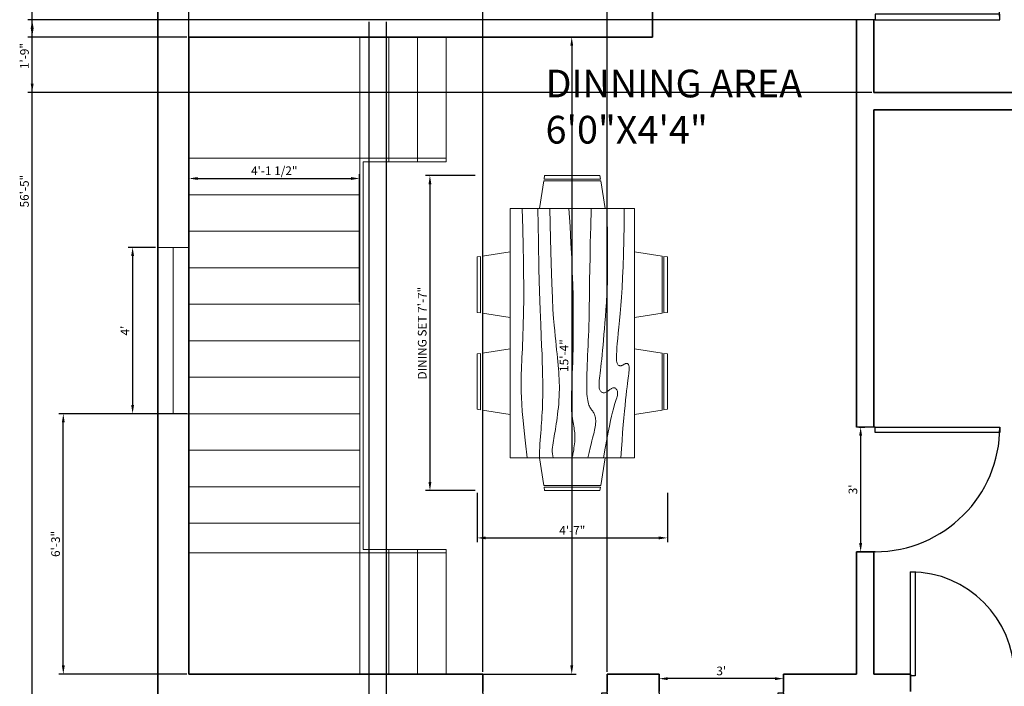
# Model space of a CAD drawing. Units: inches. Extents: x 3715 to 4224, y 2597 to 3354.
# Tile 2 of 5: x 3717 to 4001, y 2830 to 3023. Entities that reach past the tile are written whole.
import ezdxf

# ---------------------------------------------------------------- set-up
doc = ezdxf.new("R2010")
doc.units = ezdxf.units.IN
for name, color, linetype, lineweight in [('A-AREA-IDEN', 4, 'Continuous', 25), ('A-FLOR-STRS', 7, 'Continuous', 18), ('A-WALL', 7, 'Continuous', 35), ('DIM', 1, 'Continuous', 18), ('DOOR', 3, 'Continuous', 25), ('FURNITURES', 30, 'Continuous', 18), ('WINDOW', 6, 'Continuous', 20)]:
    doc.layers.add(name, color=color, linetype=linetype, lineweight=lineweight)
doc.styles.get("Standard").update_dxf_attribs({"font": 'arial.ttf'})
doc.dimstyles.new('ISO-25', dxfattribs={"dimtxt": 2.5, "dimasz": 2.5, "dimexe": 1.25, "dimexo": 0.625, "dimtad": 1, "dimlunit": 3, "dimtxsty": 'Standard', "dimcen": 2.5, "dimadec": 0, "dimazin": 0, "dimtfac": 1, "dimtmove": 0, "dimatfit": 3, "dimfxl": 1, "dimarcsym": 0})

# ---------------------------------------------------------------- blocks, each defined once
blk = doc.blocks.new('*U3')
for p, q in [((-40, 0), (-40, 6)), ((0, 0), (0, 6))]:
    blk.add_line(p, q)
blk.add_lwpolyline([(0, 0), (0, -40), (-1.75, -40), (-1.75, 0)], close=True)
blk.add_arc((0, 0), 40, 180, 270)
blk = doc.blocks.new('*U2')
for p, q in [((0, 0), (0, -6)), ((40, 0), (40, -6))]:
    blk.add_line(p, q)
blk.add_lwpolyline([(0, 0), (0, 40), (1.75, 40), (1.75, 0)], close=True)
blk.add_arc((0, 0), 40, 0, 90)
blk = doc.blocks.new('*U4')
for p, q in [((0, 0), (0, -6)), ((-40, 0), (-40, -6))]:
    blk.add_line(p, q)
blk.add_lwpolyline([(0, 0), (0, 40), (-1.75, 40), (-1.75, 0)], close=True)
blk.add_arc((0, 0), 40, 90, 180)
blk = doc.blocks.new('Dining Set - 36 x 72 in.')
for p, q in [((-22.2343, 26.00059), (-23.4847, 17.99762)), ((-22.2304, 26), (-5.7608, 26)), ((-22, 27.5), (-22.1562, 26.50042)), ((-5.8416, 26.5), (-22.1534, 26.5)), ((-22, 27.5), (-6, 27.5)), ((-5.8437, 26.49966), (-6, 27.5)), ((-4.5152, 17.99762), (-5.7655, 25.99926)), ((5.7657, 26.00059), (4.5153, 17.99762)), ((5.7696, 26), (22.2392, 26)), ((6, 27.5), (5.8438, 26.50042)), ((22.1584, 26.5), (5.8466, 26.5)), ((6, 27.5), (22, 27.5)), ((22.1563, 26.49966), (22, 27.5)), ((23.4848, 17.99762), (22.2345, 25.99926)), ((36, 18), (-36, 18)), ((-36, 18), (-36, -18)), ((36, -18), (36, 18)), ((-44.0006, 8.23428), (-35.9976, 9.48474)), ((44.0006, 8.23428), (35.9976, 9.48474)), ((-45.5, 8), (-44.5004, 8.15617)), ((-45.5, 8), (-45.5, -8)), ((-44.5, -8.15843), (-44.5, 8.15338)), ((-44, 8.23041), (-44, -8.23915)), ((44, 8.23041), (44, -8.23915)), ((44.5, -8.15843), (44.5, 8.15338)), ((45.5, 8), (44.5005, 8.15617)), ((45.5, 8), (45.5, -8)), ((-44.4997, -8.15631), (-45.5, -8)), ((-35.9976, -9.48476), (-43.9993, -8.2345)), ((35.9976, -9.48476), (43.9993, -8.2345)), ((44.4997, -8.15631), (45.5, -8)), ((-36, -18), (36, -18)), ((-22.2343, -26.0006), (-23.4847, -17.99762)), ((-4.5152, -17.99762), (-5.7655, -25.99928)), ((5.7657, -26.0006), (4.5153, -17.99762)), ((23.4848, -17.99762), (22.2345, -25.99928)), ((-22.2304, -26), (-5.7608, -26)), ((-22, -27.5), (-22.1562, -26.50044)), ((-5.8416, -26.5), (-22.1534, -26.5)), ((-22, -27.5), (-6, -27.5)), ((-5.8437, -26.49967), (-6, -27.5)), ((5.7696, -26), (22.2392, -26)), ((6, -27.5), (5.8438, -26.50044)), ((22.1584, -26.5), (5.8466, -26.5)), ((6, -27.5), (22, -27.5)), ((22.1563, -26.49967), (22, -27.5))]:
    blk.add_line(p, q)
for points in [[(-36, 15), (-31.1772, 14.97754), (-26.8079, 14.91406), (-22.8538, 14.81543), (-19.276, 14.6875), (-16.0362, 14.53613), (-13.0957, 14.36718), (-10.4159, 14.18652), (-7.9583, 14), (-5.6904, 13.81315), (-3.6035, 13.63021), (-1.6954, 13.45508), (0.0365, 13.29166), (1.5945, 13.14388), (2.9811, 13.01562), (4.1988, 12.9108), (5.25, 12.83333), (6.1393, 12.78613), (6.8802, 12.76823), (7.4883, 12.77767), (7.9792, 12.8125), (8.3685, 12.87077), (8.6719, 12.95052), (8.9049, 13.0498), (9.0833, 13.16666), (9.2205, 13.29899), (9.3216, 13.44401), (9.3895, 13.59879), (9.4271, 13.76041), (9.4373, 13.92594), (9.4232, 14.09245), (9.3875, 14.257), (9.3333, 14.41666), (9.2638, 14.56917), (9.1836, 14.71484), (9.0975, 14.85465), (9.0104, 14.98958), (8.9272, 15.1206), (8.8529, 15.2487), (8.7922, 15.37483), (8.75, 15.5), (8.7305, 15.62467), (8.7344, 15.74739), (8.7617, 15.86621), (8.8125, 15.97916), (8.8867, 16.08431), (8.9844, 16.17968), (9.1055, 16.26334), (9.25, 16.33333), (9.4189, 16.38802), (9.6172, 16.42708), (9.8506, 16.45052), (10.125, 16.45833), (10.4463, 16.45052), (10.8203, 16.42708), (11.2529, 16.38802), (11.75, 16.33333), (12.3184, 16.26318), (12.9694, 16.17838), (13.7151, 16.07991), (14.5677, 15.96875), (15.5395, 15.84586), (16.6426, 15.71224), (17.8893, 15.56884), (19.2917, 15.41666), (20.859, 15.25667), (22.5879, 15.08984), (24.4721, 14.91715), (26.5052, 14.73958), (28.6809, 14.5581), (30.9929, 14.3737), (33.4347, 14.18733), (36, 14)], [(-36, 10), (-28.9766, 10.14274), (-23.1725, 10.20442), (-18.4241, 10.19775), (-14.5677, 10.13541), (-11.4399, 10.03011), (-8.877, 9.89453), (-6.7154, 9.74137), (-4.7917, 9.58333), (-2.9698, 9.43082), (-1.2246, 9.28515), (0.4415, 9.14534), (2.026, 9.01041), (3.5266, 8.87939), (4.9408, 8.7513), (6.266, 8.62516), (7.5, 8.5), (8.6411, 8.37549), (9.6914, 8.2539), (10.6538, 8.13818), (11.5312, 8.03125), (12.3267, 7.93603), (13.043, 7.85547), (13.6831, 7.79248), (14.25, 7.75), (14.7471, 7.7303), (15.1797, 7.73307), (15.5537, 7.75732), (15.875, 7.80208), (16.1494, 7.86637), (16.3828, 7.94922), (16.5811, 8.04964), (16.75, 8.16666), (16.8944, 8.29915), (17.0143, 8.44531), (17.1089, 8.60319), (17.1771, 8.77083), (17.218, 8.94629), (17.2305, 9.1276), (17.2137, 9.31282), (17.1667, 9.5), (17.0895, 9.6875), (16.987, 9.875), (16.8649, 10.0625), (16.7292, 10.25), (16.5856, 10.4375), (16.4401, 10.625), (16.2985, 10.8125), (16.1667, 11), (16.05, 11.18733), (15.9518, 11.3737), (15.8752, 11.5581), (15.8229, 11.73958), (15.798, 11.91715), (15.8034, 12.08984), (15.842, 12.25667), (15.9167, 12.41666), (16.0295, 12.56836), (16.1784, 12.70833), (16.3605, 12.83268), (16.5729, 12.9375), (16.8127, 13.01888), (17.0768, 13.07291), (17.3625, 13.0957), (17.6667, 13.08333), (17.9894, 13.03312), (18.3418, 12.94726), (18.7382, 12.82918), (19.1927, 12.68229), (19.7195, 12.51001), (20.3327, 12.31575), (21.0465, 12.10294), (21.875, 11.875), (22.8357, 11.63354), (23.959, 11.37304), (25.2786, 11.08618), (26.8282, 10.76562), (28.6414, 10.40405), (30.752, 9.99414), (33.1936, 9.52856), (36, 9)], [(-36, 5.5), (-30.7157, 5.3348), (-26.069, 5.20963), (-21.9946, 5.11767), (-18.4271, 5.05208), (-15.3009, 5.00602), (-12.5508, 4.97265), (-10.1112, 4.94515), (-7.9167, 4.91666), (-5.909, 4.88167), (-4.0586, 4.83984), (-2.3429, 4.79215), (-0.7396, 4.73958), (0.7739, 4.6831), (2.22, 4.6237), (3.6213, 4.56233), (5, 4.5), (6.373, 4.43782), (7.7344, 4.3776), (9.0723, 4.32129), (10.375, 4.27083), (11.6309, 4.22819), (12.8281, 4.19531), (13.9551, 4.17415), (15, 4.16666), (15.954, 4.17448), (16.819, 4.19791), (17.6001, 4.23698), (18.3021, 4.29166), (18.9299, 4.36198), (19.4883, 4.44791), (19.9823, 4.54948), (20.4167, 4.66666), (20.7969, 4.79899), (21.1302, 4.94401), (21.4245, 5.09879), (21.6875, 5.26041), (21.9271, 5.42594), (22.1511, 5.59245), (22.3672, 5.757), (22.5834, 5.91666), (22.8065, 6.06868), (23.0404, 6.21093), (23.2879, 6.34147), (23.5521, 6.45833), (23.8358, 6.55957), (24.142, 6.64323), (24.4735, 6.70735), (24.8334, 6.75), (25.2235, 6.76969), (25.642, 6.76692), (26.0858, 6.74267), (26.5521, 6.69791), (27.0379, 6.63362), (27.5404, 6.55078), (28.0565, 6.45036), (28.5834, 6.33333), (29.1242, 6.19987), (29.7071, 6.04687), (30.3661, 5.87044), (31.1354, 5.66666), (32.0493, 5.43164), (33.142, 5.16146), (34.4475, 4.85221), (36, 4.5)], [(-36, -1), (-30.7915, -0.6591), (-26.0195, -0.38216), (-21.6519, -0.16284), (-17.6563, 0.00521), (-14.0005, 0.12833), (-10.6523, 0.21289), (-7.5796, 0.26522), (-4.75, 0.29166), (-2.134, 0.29793), (0.2878, 0.28711), (2.5317, 0.26163), (4.6146, 0.22396), (6.5529, 0.17651), (8.3633, 0.12174), (10.0623, 0.06209), (11.6667, 0), (13.1899, -0.06201), (14.6341, -0.1211), (15.9982, -0.17432), (17.2813, -0.21875), (18.4823, -0.25147), (19.6003, -0.26953), (20.6343, -0.27002), (21.5834, -0.25), (22.4481, -0.20768), (23.2357, -0.14584), (23.9549, -0.06836), (24.6146, 0.02083), (25.2235, 0.11784), (25.7904, 0.21875), (26.3241, 0.31966), (26.8334, 0.41666), (27.3265, 0.50618), (27.8099, 0.58593), (28.2894, 0.65397), (28.7709, 0.70833), (29.2601, 0.74707), (29.763, 0.76823), (30.2855, 0.76985), (30.8334, 0.75), (31.4088, 0.70784), (31.9994, 0.64713), (32.589, 0.57275), (33.1615, 0.48958), (33.7008, 0.4025), (34.1908, 0.3164), (34.6153, 0.23616), (34.9584, 0.16666), (35.2099, 0.11165), (35.3848, 0.07031), (35.504, 0.04069), (35.5886, 0.02083), (35.6594, 0.00879), (35.7377, 0.0026), (35.8442, 0.00032), (36, 0)], [(-36, -6.5), (-27.1843, -6.31267), (-20.084, -6.1263), (-14.469, -5.9419), (-10.1094, -5.76042), (-6.7752, -5.58285), (-4.2363, -5.41016), (-2.2629, -5.24333), (-0.625, -5.08334), (0.8708, -4.93099), (2.2715, -4.78646), (3.5872, -4.64974), (4.8281, -4.52084), (6.0046, -4.39974), (7.127, -4.28646), (8.2053, -4.18099), (9.25, -4.08334), (10.2705, -3.99382), (11.2734, -3.91407), (12.2647, -3.84603), (13.25, -3.79167), (14.2354, -3.75293), (15.2266, -3.73177), (16.2295, -3.73015), (17.25, -3.75), (18.2912, -3.79248), (19.3451, -3.85547), (20.4009, -3.93604), (21.4479, -4.03125), (22.4754, -4.13819), (23.4727, -4.25391), (24.4289, -4.37549), (25.3334, -4.5), (26.1785, -4.62492), (26.9694, -4.74935), (27.7145, -4.87281), (28.4219, -4.99479), (29.1, -5.11483), (29.7572, -5.23242), (30.4016, -5.34709), (31.0417, -5.45834), (31.6837, -5.56437), (32.3262, -5.65821), (32.9658, -5.73153), (33.599, -5.77604), (34.2224, -5.78345), (34.8327, -5.74545), (35.4264, -5.65373), (36, -5.5)], [(-36, -10), (-26.4022, -9.81299), (-18.4675, -9.62891), (-11.9839, -9.45069), (-6.7396, -9.28125), (-2.5226, -9.12354), (0.8789, -8.98047), (3.6769, -8.85498), (6.0833, -8.75), (8.2767, -8.66765), (10.3021, -8.60677), (12.1712, -8.56543), (13.8958, -8.54167), (15.4876, -8.53353), (16.9583, -8.53907), (18.3197, -8.55632), (19.5834, -8.58334), (20.7616, -8.61841), (21.8685, -8.66081), (22.9188, -8.71004), (23.9271, -8.76563), (24.9081, -8.82707), (25.8763, -8.89388), (26.8465, -8.96558), (27.8334, -9.04167), (28.8474, -9.12118), (29.8828, -9.20117), (30.93, -9.27824), (31.9792, -9.34896), (33.0205, -9.40991), (34.0443, -9.45768), (35.0407, -9.48885), (36, -9.5)], [(-36, -14.5), (-30.0881, -14.33513), (-25.0332, -14.21224), (-20.7312, -14.12647), (-17.0781, -14.07292), (-13.97, -14.04671), (-11.3027, -14.04297), (-8.9724, -14.05681), (-6.875, -14.08334), (-4.9224, -14.11833), (-3.0905, -14.16016), (-1.3709, -14.20785), (0.2448, -14.26042), (1.7647, -14.3169), (3.1973, -14.3763), (4.5507, -14.43767), (5.8333, -14.5), (7.0554, -14.5621), (8.235, -14.62175), (9.3922, -14.67652), (10.5469, -14.72396), (11.7192, -14.76164), (12.929, -14.78711), (14.1965, -14.79794), (15.5417, -14.79167), (16.9933, -14.76424), (18.6152, -14.70508), (20.4804, -14.60197), (22.6615, -14.44271), (25.2312, -14.21509), (28.2624, -13.9069), (31.8277, -13.50594), (36, -13)]]:
    blk.add_lwpolyline(points)
blk = doc.blocks.new('*D25')
at = {"layer": 'Defpoints', "color": 0, "transparency": 16777216}
for p in [(3756.48, 2957.15), (3749.21, 2909.15), (3756.48, 2909.15)]:
    blk.add_point(p, dxfattribs=at)
at = {"layer": 'DIM', "color": 0, "lineweight": -2, "transparency": 16777216}
for p, q in [((3755.85, 2957.15), (3747.96, 2957.15)), ((3749.21, 2954.65), (3749.21, 2911.65)), ((3755.85, 2909.15), (3747.96, 2909.15))]:
    blk.add_line(p, q, dxfattribs=at)
at = {"layer": 'DIM', "color": 0, "transparency": 16777216}
for points in [[(3748.79, 2954.65), (3749.63, 2954.65), (3749.21, 2957.15)], [(3748.79, 2911.65), (3749.63, 2911.65), (3749.21, 2909.15)]]:
    blk.add_solid(points, dxfattribs=at)
at = {"layer": 'DIM', "color": 0, "transparency": 16777216, "insert": (3747.34, 2933.15), "char_height": 2.5, "attachment_point": 5, "rotation": 90}
blk.add_mtext("4'", dxfattribs=at)
blk = doc.blocks.new('*D34')
at = {"layer": 'Defpoints', "color": 0, "transparency": 16777216}
for p in [(3958.48, 2905.29), (3958.68, 2869.29), (3959.65, 2869.29)]:
    blk.add_point(p, dxfattribs=at)
at = {"layer": 'DIM', "color": 0, "lineweight": -2, "transparency": 16777216}
for p, q in [((3959.1, 2905.29), (3960.9, 2905.29)), ((3959.65, 2902.79), (3959.65, 2871.79)), ((3959.3, 2869.29), (3960.9, 2869.29))]:
    blk.add_line(p, q, dxfattribs=at)
at = {"layer": 'DIM', "color": 0, "transparency": 16777216}
for points in [[(3959.23, 2902.79), (3960.07, 2902.79), (3959.65, 2905.29)], [(3959.23, 2871.79), (3960.07, 2871.79), (3959.65, 2869.29)]]:
    blk.add_solid(points, dxfattribs=at)
at = {"layer": 'DIM', "color": 0, "transparency": 16777216, "insert": (3957.75, 2887.29), "char_height": 2.5, "attachment_point": 5, "rotation": 90}
blk.add_mtext("3'", dxfattribs=at)
blk = doc.blocks.new('*D36')
at = {"layer": 'Defpoints', "color": 0, "transparency": 16777216}
for p in [(3901.38, 2833.93), (3901.38, 2832.63), (3937.38, 2833.93)]:
    blk.add_point(p, dxfattribs=at)
at = {"layer": 'DIM', "color": 0, "lineweight": -2, "transparency": 16777216}
for p, q in [((3901.38, 2833.31), (3901.38, 2831.38)), ((3934.88, 2832.63), (3903.88, 2832.63)), ((3937.38, 2833.31), (3937.38, 2831.38))]:
    blk.add_line(p, q, dxfattribs=at)
at = {"layer": 'DIM', "color": 0, "transparency": 16777216}
for points in [[(3903.88, 2833.05), (3903.88, 2832.21), (3901.38, 2832.63)], [(3934.88, 2833.05), (3934.88, 2832.21), (3937.38, 2832.63)]]:
    blk.add_solid(points, dxfattribs=at)
at = {"layer": 'DIM', "color": 0, "transparency": 16777216, "insert": (3919.38, 2834.53), "char_height": 2.5, "attachment_point": 5}
blk.add_mtext("3'", dxfattribs=at)
blk = doc.blocks.new('WIN-48IN-9IN-WALL')
blk.add_line((4.5, 48), (4.5, 0))
blk.add_lwpolyline([(0, 48), (9, 48), (9, 0), (0, 0)], close=True)
blk = doc.blocks.new('*D59')
at = {"layer": 'Defpoints', "color": 0, "transparency": 16777216}
for p in [(3848.8, 2977.92), (3835.15, 2886.92), (3848.8, 2886.92)]:
    blk.add_point(p, dxfattribs=at)
at = {"layer": 'DIM', "color": 0, "lineweight": -2, "transparency": 16777216}
for p, q in [((3848.18, 2977.92), (3833.9, 2977.92)), ((3835.15, 2975.42), (3835.15, 2889.42)), ((3848.18, 2886.92), (3833.9, 2886.92))]:
    blk.add_line(p, q, dxfattribs=at)
at = {"layer": 'DIM', "color": 0, "transparency": 16777216}
for points in [[(3834.74, 2975.42), (3835.57, 2975.42), (3835.15, 2977.92)], [(3834.74, 2889.42), (3835.57, 2889.42), (3835.15, 2886.92)]]:
    blk.add_solid(points, dxfattribs=at)
at = {"layer": 'DIM', "color": 0, "transparency": 16777216, "insert": (3833.24, 2932.42), "char_height": 2.5, "attachment_point": 5, "rotation": 90}
blk.add_mtext('DINING SET 7\'-7"', dxfattribs=at)
blk = doc.blocks.new('*D60')
at = {"layer": 'Defpoints', "color": 0, "transparency": 16777216}
for p in [(3848.8, 2886.92), (3903.8, 2886.92), (3903.8, 2873.27)]:
    blk.add_point(p, dxfattribs=at)
at = {"layer": 'DIM', "color": 0, "lineweight": -2, "transparency": 16777216}
for p, q in [((3848.8, 2886.3), (3848.8, 2872.02)), ((3903.8, 2886.3), (3903.8, 2872.02)), ((3851.3, 2873.27), (3901.3, 2873.27))]:
    blk.add_line(p, q, dxfattribs=at)
at = {"layer": 'DIM', "color": 0, "transparency": 16777216}
for points in [[(3851.3, 2873.69), (3851.3, 2872.85), (3848.8, 2873.27)], [(3901.3, 2873.69), (3901.3, 2872.85), (3903.8, 2873.27)]]:
    blk.add_solid(points, dxfattribs=at)
at = {"layer": 'DIM', "color": 0, "transparency": 16777216, "insert": (3876.3, 2875.15), "char_height": 2.5, "attachment_point": 5}
blk.add_mtext('4\'-7"', dxfattribs=at)
blk = doc.blocks.new('*D76')
at = {"layer": 'Defpoints', "color": 0, "transparency": 16777216}
for p in [(3720.18, 3311.93), (3756.48, 3311.93), (3756.48, 2634.93)]:
    blk.add_point(p, dxfattribs=at)
at = {"layer": 'DIM', "color": 0, "lineweight": -2, "transparency": 16777216}
for p, q in [((3755.85, 3311.93), (3718.93, 3311.93)), ((3720.18, 2637.43), (3720.18, 3309.43)), ((3755.85, 2634.93), (3718.93, 2634.93))]:
    blk.add_line(p, q, dxfattribs=at)
at = {"layer": 'DIM', "color": 0, "transparency": 16777216}
for points in [[(3719.76, 3309.43), (3720.59, 3309.43), (3720.18, 3311.93)], [(3719.76, 2637.43), (3720.59, 2637.43), (3720.18, 2634.93)]]:
    blk.add_solid(points, dxfattribs=at)
at = {"layer": 'DIM', "color": 0, "transparency": 16777216, "insert": (3718.27, 2973.43), "char_height": 2.5, "attachment_point": 5, "rotation": 90}
blk.add_mtext('56\'-5"', dxfattribs=at)
blk = doc.blocks.new('*D79')
at = {"layer": 'Defpoints', "color": 0, "transparency": 16777216}
for p in [(3720.18, 3136.93), (3765.48, 3136.93), (3765.48, 3017.93)]:
    blk.add_point(p, dxfattribs=at)
at = {"layer": 'DIM', "color": 0, "lineweight": -2, "transparency": 16777216}
for p, q in [((3764.85, 3136.93), (3718.93, 3136.93)), ((3720.18, 3020.43), (3720.18, 3134.43)), ((3764.85, 3017.93), (3718.93, 3017.93))]:
    blk.add_line(p, q, dxfattribs=at)
at = {"layer": 'DIM', "color": 0, "transparency": 16777216}
for points in [[(3719.76, 3134.43), (3720.59, 3134.43), (3720.18, 3136.93)], [(3719.76, 3020.43), (3720.59, 3020.43), (3720.18, 3017.93)]]:
    blk.add_solid(points, dxfattribs=at)
at = {"layer": 'DIM', "color": 0, "transparency": 16777216, "insert": (3718.27, 3077.43), "char_height": 2.5, "attachment_point": 5, "rotation": 90}
blk.add_mtext('9\'-11"', dxfattribs=at)
blk = doc.blocks.new('*D80')
at = {"layer": 'Defpoints', "color": 0, "transparency": 16777216}
for p in [(3814.84, 2977.07), (3765.48, 2940.77), (3814.84, 2940.77)]:
    blk.add_point(p, dxfattribs=at)
at = {"layer": 'DIM', "color": 0, "lineweight": -2, "transparency": 16777216}
for p, q in [((3765.48, 2941.4), (3765.48, 2978.32)), ((3767.98, 2977.07), (3812.34, 2977.07)), ((3814.84, 2941.4), (3814.84, 2978.32))]:
    blk.add_line(p, q, dxfattribs=at)
at = {"layer": 'DIM', "color": 0, "transparency": 16777216}
for points in [[(3767.98, 2977.49), (3767.98, 2976.66), (3765.48, 2977.07)], [(3812.34, 2977.49), (3812.34, 2976.66), (3814.84, 2977.07)]]:
    blk.add_solid(points, dxfattribs=at)
at = {"layer": 'DIM', "color": 0, "transparency": 16777216, "insert": (3790.16, 2978.99), "char_height": 2.5, "attachment_point": 5}
blk.add_mtext('4\'-1 1/2"', dxfattribs=at)
blk = doc.blocks.new('*D83')
at = {"layer": 'Defpoints', "color": 0, "transparency": 16777216}
for p in [(3850.41, 3348.23), (3765.48, 2833.93), (3850.41, 2833.93)]:
    blk.add_point(p, dxfattribs=at)
at = {"layer": 'DIM', "color": 0, "lineweight": -2, "transparency": 16777216}
for p, q in [((3765.48, 2834.56), (3765.48, 3349.48)), ((3767.98, 3348.23), (3847.91, 3348.23)), ((3850.41, 2834.56), (3850.41, 3349.48))]:
    blk.add_line(p, q, dxfattribs=at)
at = {"layer": 'DIM', "color": 0, "transparency": 16777216}
for points in [[(3767.98, 3348.65), (3767.98, 3347.82), (3765.48, 3348.23)], [(3847.91, 3348.65), (3847.91, 3347.82), (3850.41, 3348.23)]]:
    blk.add_solid(points, dxfattribs=at)
at = {"layer": 'DIM', "color": 0, "transparency": 16777216, "insert": (3807.94, 3350.11), "char_height": 2.5, "attachment_point": 5}
blk.add_mtext('7\'-1"', dxfattribs=at)
blk = doc.blocks.new('*D84')
at = {"layer": 'Defpoints', "color": 0, "transparency": 16777216}
for p in [(3886.41, 3348.23), (3850.41, 2833.93), (3886.41, 2833.93)]:
    blk.add_point(p, dxfattribs=at)
at = {"layer": 'DIM', "color": 0, "lineweight": -2, "transparency": 16777216}
for p, q in [((3850.41, 2834.56), (3850.41, 3349.48)), ((3852.91, 3348.23), (3883.91, 3348.23)), ((3886.41, 2834.56), (3886.41, 3349.48))]:
    blk.add_line(p, q, dxfattribs=at)
at = {"layer": 'DIM', "color": 0, "transparency": 16777216}
for points in [[(3852.91, 3348.65), (3852.91, 3347.82), (3850.41, 3348.23)], [(3883.91, 3348.65), (3883.91, 3347.82), (3886.41, 3348.23)]]:
    blk.add_solid(points, dxfattribs=at)
at = {"layer": 'DIM', "color": 0, "transparency": 16777216, "insert": (3868.41, 3350.14), "char_height": 2.5, "attachment_point": 5}
blk.add_mtext('3\'-0"', dxfattribs=at)
blk = doc.blocks.new('*D85')
at = {"layer": 'Defpoints', "color": 0, "transparency": 16777216}
for p in [(3817.48, 3022.93), (3822.48, 3022.93), (3822.48, 2598.63)]:
    blk.add_point(p, dxfattribs=at)
at = {"layer": 'DIM', "color": 0, "lineweight": -2, "transparency": 16777216}
for p, q in [((3817.48, 3022.31), (3817.48, 2597.38)), ((3822.48, 3022.31), (3822.48, 2597.38)), ((3814.98, 2598.63), (3812.48, 2598.63)), ((3817.48, 2598.63), (3822.48, 2598.63)), ((3824.98, 2598.63), (3835.37, 2598.63))]:
    blk.add_line(p, q, dxfattribs=at)
at = {"layer": 'DIM', "color": 0, "transparency": 16777216}
for points in [[(3814.98, 2599.05), (3814.98, 2598.22), (3817.48, 2598.63)], [(3824.98, 2599.05), (3824.98, 2598.22), (3822.48, 2598.63)]]:
    blk.add_solid(points, dxfattribs=at)
at = {"layer": 'DIM', "color": 0, "transparency": 16777216, "insert": (3831.42, 2600.54), "char_height": 2.5, "attachment_point": 5}
blk.add_mtext('0\'-5"', dxfattribs=at)
blk = doc.blocks.new('*D90')
at = {"layer": 'Defpoints', "color": 0, "transparency": 16777216}
for p in [(3720.18, 3022.93), (3963.48, 3022.93), (3963.48, 3001.93)]:
    blk.add_point(p, dxfattribs=at)
at = {"layer": 'DIM', "color": 0, "lineweight": -2, "transparency": 16777216}
for p, q in [((3962.85, 3022.93), (3718.93, 3022.93)), ((3720.18, 3004.43), (3720.18, 3020.43)), ((3962.85, 3001.93), (3718.93, 3001.93))]:
    blk.add_line(p, q, dxfattribs=at)
at = {"layer": 'DIM', "color": 0, "transparency": 16777216}
for points in [[(3719.76, 3020.43), (3720.59, 3020.43), (3720.18, 3022.93)], [(3719.76, 3004.43), (3720.59, 3004.43), (3720.18, 3001.93)]]:
    blk.add_solid(points, dxfattribs=at)
at = {"layer": 'DIM', "color": 0, "transparency": 16777216, "insert": (3718.27, 3012.43), "char_height": 2.5, "attachment_point": 5, "rotation": 90}
blk.add_mtext('1\'-9"', dxfattribs=at)
blk = doc.blocks.new('*D99')
at = {"layer": 'Defpoints', "color": 0, "transparency": 16777216}
for p in [(3839.84, 3017.93), (3839.84, 2833.93), (3876.14, 2833.93)]:
    blk.add_point(p, dxfattribs=at)
at = {"layer": 'DIM', "color": 0, "lineweight": -2, "transparency": 16777216}
for p, q in [((3840.47, 3017.93), (3877.39, 3017.93)), ((3876.14, 3015.43), (3876.14, 2836.43)), ((3840.47, 2833.93), (3877.39, 2833.93))]:
    blk.add_line(p, q, dxfattribs=at)
at = {"layer": 'DIM', "color": 0, "transparency": 16777216}
for points in [[(3875.73, 3015.43), (3876.56, 3015.43), (3876.14, 3017.93)], [(3875.73, 2836.43), (3876.56, 2836.43), (3876.14, 2833.93)]]:
    blk.add_solid(points, dxfattribs=at)
at = {"layer": 'DIM', "color": 0, "transparency": 16777216, "insert": (3874.24, 2925.93), "char_height": 2.5, "attachment_point": 5, "rotation": 90}
blk.add_mtext('15\'-4"', dxfattribs=at)
blk = doc.blocks.new('*D101')
at = {"layer": 'Defpoints', "color": 0, "transparency": 16777216}
for p in [(3729.18, 2909.15), (3765.48, 2909.15), (3765.48, 2833.93)]:
    blk.add_point(p, dxfattribs=at)
at = {"layer": 'DIM', "color": 0, "lineweight": -2, "transparency": 16777216}
for p, q in [((3764.85, 2909.15), (3727.93, 2909.15)), ((3729.18, 2836.43), (3729.18, 2906.65)), ((3764.85, 2833.93), (3727.93, 2833.93))]:
    blk.add_line(p, q, dxfattribs=at)
at = {"layer": 'DIM', "color": 0, "transparency": 16777216}
for points in [[(3728.76, 2906.65), (3729.59, 2906.65), (3729.18, 2909.15)], [(3728.76, 2836.43), (3729.59, 2836.43), (3729.18, 2833.93)]]:
    blk.add_solid(points, dxfattribs=at)
at = {"layer": 'DIM', "color": 0, "transparency": 16777216, "insert": (3727.27, 2871.54), "char_height": 2.5, "attachment_point": 5, "rotation": 90}
blk.add_mtext('6\'-3"', dxfattribs=at)

msp = doc.modelspace()

# ---------------------------------------------------------------- linework, layer by layer
at = {"layer": 'A-FLOR-STRS'}
for p, q in [((3814.843, 2982.934), (3814.843, 3017.934)), ((3823.262, 2981.934), (3823.262, 3017.934)), ((3823.262, 3017.934), (3823.262, 2981.934)), ((3823.262, 3017.934), (3823.262, 2981.934)), ((3831.553, 2981.934), (3831.553, 3017.934)), ((3831.553, 3017.934), (3831.553, 2981.934)), ((3831.553, 3017.934), (3831.553, 2981.934)), ((3839.843, 3017.934), (3839.843, 2981.934)), ((3839.843, 3017.934), (3839.843, 2981.934)), ((3839.843, 2981.934), (3839.843, 3017.934)), ((3814.843, 2982.934), (3765.476, 2982.934)), ((3814.843, 2972.393), (3765.476, 2972.393)), ((3814.843, 2961.853), (3765.476, 2961.853)), ((3814.843, 2951.313), (3765.476, 2951.313)), ((3814.843, 2940.773), (3765.476, 2940.773)), ((3814.843, 2930.232), (3765.476, 2930.232)), ((3814.843, 2919.692), (3765.476, 2919.692)), ((3814.843, 2909.152), (3765.476, 2909.152)), ((3814.843, 2898.612), (3765.476, 2898.612)), ((3814.843, 2888.071), (3765.476, 2888.071)), ((3814.843, 2877.531), (3765.476, 2877.531)), ((3814.843, 2868.934), (3765.476, 2868.934)), ((3814.843, 2868.934), (3814.843, 2833.934)), ((3823.262, 2869.934), (3823.262, 2833.934)), ((3823.262, 2833.934), (3823.262, 2869.934)), ((3823.262, 2833.934), (3823.262, 2869.934)), ((3831.553, 2869.934), (3831.553, 2833.934)), ((3831.553, 2833.934), (3831.553, 2869.934)), ((3831.553, 2833.934), (3831.553, 2869.934)), ((3839.843, 2833.934), (3839.843, 2869.934))]:
    msp.add_line(p, q, dxfattribs=at)
for points in [[(3839.843, 2982.934), (3814.843, 2982.934), (3814.843, 2868.934), (3839.843, 2868.934)], [(3839.843, 2981.934), (3815.843, 2981.934), (3815.843, 2869.934), (3839.843, 2869.934)]]:
    msp.add_lwpolyline(points, dxfattribs=at)
at = {"layer": 'A-WALL'}
for p, q in [((3756.476, 2634.934), (3756.476, 3311.934)), ((3899.476, 3017.934), (3899.476, 3032.26)), ((3958.476, 2905.291), (3958.476, 3022.934)), ((3963.476, 3001.934), (3963.476, 3022.934)), ((3765.476, 3017.934), (3899.476, 3017.934)), ((3765.476, 2833.934), (3765.476, 3017.934)), ((3963.476, 3001.934), (4185.476, 3001.934)), ((3963.476, 2996.934), (4185.476, 2996.934)), ((3963.476, 2905.291), (3963.476, 2996.934)), ((3958.476, 2833.934), (3958.476, 2869.291)), ((3963.476, 2833.934), (3963.476, 2869.291)), ((3765.476, 2833.934), (3850.407, 2833.934)), ((3886.407, 2833.934), (3901.381, 2833.934)), ((3937.381, 2833.934), (3958.476, 2833.934)), ((3963.476, 2833.934), (3974.058, 2833.934))]:
    msp.add_line(p, q, dxfattribs=at)
for points in [[(3958.676, 2869.291), (3963.676, 2869.291)], [(3850.407, 2828.934), (3850.407, 2833.934)], [(3886.407, 2833.934), (3886.407, 2828.934)], [(3901.381, 2828.934), (3901.381, 2833.934)], [(3937.381, 2833.934), (3937.381, 2828.934)], [(3974.058, 2828.934), (3974.058, 2833.934)]]:
    msp.add_lwpolyline(points, dxfattribs=at)

# ---------------------------------------------------------------- block references
at = {"layer": 'DOOR', "xscale": 0.9, "yscale": 0.9, "zscale": 0.9, "rotation": 270}
for name, p in [('*U4', (3963.876, 3022.934)), ('*U2', (3963.876, 2905.291))]:
    msp.add_blockref(name, p, dxfattribs=at)
at = {"layer": 'DOOR'}
for name, p, xscale, yscale, zscale in [('*U2', (3974.058, 2833.434), 0.75, 0.75, 0.75), ('*U3', (3886.407, 2828.534), 0.9, 0.9, 0.9), ('*U3', (3937.381, 2828.534), 0.9, 0.9, 0.9)]:
    msp.add_blockref(name, p, dxfattribs=dict(at, xscale=xscale, yscale=yscale, zscale=zscale))
at = {"layer": 'FURNITURES', "rotation": 270}
msp.add_blockref('Dining Set - 36 x 72 in.', (3876.304, 2932.421), dxfattribs=at)
at = {"layer": 'WINDOW'}
msp.add_blockref('WIN-48IN-9IN-WALL', (3756.476, 2909.152), dxfattribs=at)

# ---------------------------------------------------------------- texts
at = {"layer": 'A-AREA-IDEN', "insert": (3868.576, 3008.506), "char_height": 8, "attachment_point": 1}
msp.add_mtext_dynamic_manual_height_columns('DINNING AREA \\P6\'0"X4\'4"', width=94.29963, gutter_width=12.5, heights=[0], dxfattribs=at)

# ---------------------------------------------------------------- dimensions: what is measured, and where the dimension line sits
at = {"layer": 'DIM'}
for base, p1, p2, override, picture, middle in [((3850.407, 3348.234), (3765.476, 2833.934), (3850.407, 2833.934), {"dimdec": 1, "dimlfac": 1, "dimrnd": 0, "dimzin": 1, "dimdsep": 46, "dimlunit": 4, "dimfrac": 2}, '*D83', (3807.941, 3350.114)), ((3886.407, 3348.234), (3850.407, 2833.934), (3886.407, 2833.934), {"dimdec": 1, "dimlfac": 1, "dimrnd": 0, "dimzin": 1, "dimdsep": 46, "dimlunit": 4, "dimfrac": 2}, '*D84', (3868.407, 3350.136)), ((3822.476, 2598.634), (3817.476, 3022.934), (3822.476, 3022.934), {"dimdec": 1, "dimlfac": 1, "dimrnd": 0, "dimzin": 1, "dimdsep": 46, "dimlunit": 4, "dimfrac": 2}, '*D85', (3831.423, 2600.535)), ((3814.843, 2977.073), (3765.476, 2940.773), (3814.843, 2940.773), {"dimdec": 1, "dimlfac": 1, "dimrnd": 0, "dimzin": 1, "dimdsep": 46, "dimlunit": 4, "dimfrac": 2}, '*D80', (3790.159, 2978.99)), ((3903.804, 2873.271), (3848.804, 2886.921), (3903.804, 2886.921), {"dimdec": 1, "dimlfac": 1, "dimrnd": 0, "dimzin": 1, "dimdsep": 46, "dimlunit": 4, "dimfrac": 2}, '*D60', (3876.304, 2875.146)), ((3901.381, 2832.631), (3937.381, 2833.934), (3901.381, 2833.934), {"dimclrd": 0, "dimclre": 0, "dimclrt": 0}, '*D36', (3919.381, 2834.533))]:
    dim = msp.add_linear_dim(base=base, p1=p1, p2=p2, dimstyle='ISO-25', override=override, dxfattribs=at)
    dim.commit()
    dim.dimension.update_dxf_attribs({"geometry": picture, "text_midpoint": middle})
for base, p1, p2, angle, override, picture, middle in [((3720.176, 3311.934), (3756.476, 2634.934), (3756.476, 3311.934), 90, {"dimdec": 1, "dimlfac": 1, "dimrnd": 0, "dimzin": 1, "dimdsep": 46, "dimlunit": 4, "dimfrac": 2}, '*D76', (3718.274, 2973.434)), ((3720.176, 3136.934), (3765.476, 3017.934), (3765.476, 3136.934), 90, {"dimdec": 1, "dimlfac": 1, "dimrnd": 0, "dimzin": 1, "dimdsep": 46, "dimlunit": 4, "dimfrac": 2}, '*D79', (3718.274, 3077.434)), ((3720.176, 3022.934), (3963.476, 3001.934), (3963.476, 3022.934), 90, {"dimdec": 1, "dimlfac": 1, "dimrnd": 0, "dimzin": 1, "dimdsep": 46, "dimlunit": 4, "dimfrac": 2}, '*D90', (3718.274, 3012.434)), ((3876.143, 2833.934), (3839.843, 3017.934), (3839.843, 2833.934), 270, {"dimdec": 1, "dimlfac": 1, "dimrnd": 0, "dimzin": 1, "dimdsep": 46, "dimlunit": 4, "dimfrac": 2}, '*D99', (3874.242, 2925.934)), ((3749.211, 2909.152), (3756.476, 2957.152), (3756.476, 2909.152), 90, {"dimclrd": 0, "dimclre": 0, "dimclrt": 0}, '*D25', (3747.336, 2933.152)), ((3729.176, 2909.152), (3765.476, 2833.934), (3765.476, 2909.152), 90, {"dimdec": 1, "dimlfac": 1, "dimrnd": 0, "dimzin": 1, "dimdsep": 46, "dimlunit": 4, "dimfrac": 2}, '*D101', (3727.273, 2871.543)), ((3959.648, 2869.291), (3958.476, 2905.291), (3958.676, 2869.291), 90, {"dimclrd": 0, "dimclre": 0, "dimclrt": 0}, '*D34', (3957.746, 2887.291))]:
    dim = msp.add_linear_dim(base=base, p1=p1, p2=p2, angle=angle, dimstyle='ISO-25', override=override, dxfattribs=at)
    dim.commit()
    dim.dimension.update_dxf_attribs({"geometry": picture, "text_midpoint": middle})
dim = msp.add_linear_dim(base=(3835.154, 2886.921), p1=(3848.804, 2977.921), p2=(3848.804, 2886.921), angle=270, text='DINING SET <>', dimstyle='ISO-25', override={"dimdec": 1, "dimlfac": 1, "dimrnd": 0, "dimzin": 1, "dimdsep": 46, "dimlunit": 4, "dimfrac": 2}, dxfattribs=at)
dim.commit()
dim.dimension.update_dxf_attribs({"geometry": '*D59', "text_midpoint": (3833.237, 2932.421)})

doc.saveas('drawing.dxf')
